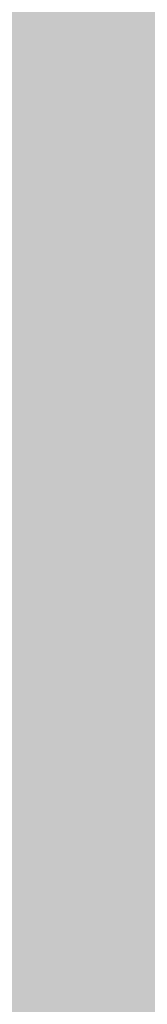
# Model space of a CAD drawing. Units: inches. Extents: x 2083 to 3317, y 1141 to 2115.
# Tile 217 of 256: x 3126.67 to 3126.939, y 1265.165 to 1267.234. Entities that reach past the tile are written whole.
import ezdxf

# ---------------------------------------------------------------- set-up
doc = ezdxf.new("R2010")
doc.units = ezdxf.units.IN
doc.layers.add('A-ANNO-DIMS', color=2, linetype='Continuous', lineweight=18)
doc.layers.add('A-WALL-PATT', color=251, linetype='Continuous', lineweight=13, true_color=0x636466)
doc.styles.get("Standard").update_dxf_attribs({"font": 'arial.ttf'})
doc.dimstyles.new('ISO-25', dxfattribs={"dimtxt": 12, "dimasz": 12, "dimexe": 1.25, "dimexo": 0.625, "dimtad": 1, "dimlunit": 3, "dimtxsty": 'Standard', "dimcen": 2.5, "dimadec": 0, "dimazin": 0, "dimtfac": 1, "dimtmove": 0, "dimatfit": 3, "dimfxl": 1, "dimarcsym": 0})

# ---------------------------------------------------------------- blocks, each defined once
blk = doc.blocks.new('*D26')
at = {"layer": 'A-ANNO-DIMS', "color": 0, "lineweight": -2, "transparency": 16777216}
for p, q in [((3088.9858, 1274.9151), (3088.9858, 1270.952)), ((3111.24, 1274.9151), (3111.24, 1270.952)), ((3076.9858, 1272.202), (2840.2624, 1272.202)), ((3111.24, 1272.202), (3088.9858, 1272.202)), ((3123.24, 1272.202), (3135.24, 1272.202))]:
    blk.add_line(p, q, dxfattribs=at)
at = {"layer": 'A-ANNO-DIMS', "color": 0, "transparency": 16777216}
for points in [[(3076.9858, 1274.202), (3076.9858, 1270.202), (3088.9858, 1272.202)], [(3123.24, 1274.202), (3123.24, 1270.202), (3111.24, 1272.202)]]:
    blk.add_solid(points, dxfattribs=at)
at = {"layer": 'Defpoints', "color": 0, "transparency": 16777216}
for p in [(3088.9858, 1275.5401), (3111.24, 1275.5401), (3088.9858, 1272.202)]:
    blk.add_point(p, dxfattribs=at)
at = {"layer": 'A-ANNO-DIMS', "color": 0, "transparency": 16777216, "insert": (2952.6241, 1279.0316), "char_height": 12, "attachment_point": 5}
blk.add_mtext('NIGHTSTAND 1\'-10 1/2" TYP.', dxfattribs=at)
blk = doc.blocks.new('*D27')
at = {"layer": 'A-ANNO-DIMS', "color": 0, "lineweight": -2, "transparency": 16777216}
for p, q in [((3114.5782, 1309.7943), (3114.5782, 1321.7943)), ((3111.865, 1297.7943), (3115.8282, 1297.7943)), ((3114.5782, 1297.7943), (3114.5782, 1275.5401)), ((3111.865, 1275.5401), (3115.8282, 1275.5401)), ((3114.5782, 1263.5401), (3114.5782, 1140.9886))]:
    blk.add_line(p, q, dxfattribs=at)
at = {"layer": 'A-ANNO-DIMS', "color": 0, "transparency": 16777216}
for points in [[(3112.5782, 1309.7943), (3116.5782, 1309.7943), (3114.5782, 1297.7943)], [(3112.5782, 1263.5401), (3116.5782, 1263.5401), (3114.5782, 1275.5401)]]:
    blk.add_solid(points, dxfattribs=at)
at = {"layer": 'Defpoints', "color": 0, "transparency": 16777216}
for p in [(3111.24, 1297.7943), (3111.24, 1275.5401), (3114.5782, 1275.5401)]:
    blk.add_point(p, dxfattribs=at)
at = {"layer": 'A-ANNO-DIMS', "color": 0, "transparency": 16777216, "insert": (3107.7485, 1196.2643), "char_height": 12, "attachment_point": 5, "rotation": 90}
blk.add_mtext('1\'-10 1/2" TYP.', dxfattribs=at)

msp = doc.modelspace()

# ---------------------------------------------------------------- hatches: boundary and pattern name
at = {"layer": 'A-WALL-PATT'}
h = msp.add_hatch(color=256, dxfattribs=at)
h.dxf.hatch_style = 1
h.paths.add_polyline_path([(3126.9598, 2020.7614), (2748.9598, 2020.7614), (2604.9598, 2020.7614), (2226.9598, 2020.7614), (2226.9598, 1702.7614), (2466.9598, 1702.7614), (2466.9598, 1582.7614), (2418.9598, 1582.7614), (2418.9598, 1477.7614), (2226.9598, 1477.7614), (2226.9598, 1263.2614), (2544.9598, 1263.2614), (2544.9598, 1411.7614), (2604.9598, 1411.7614), (2685.9598, 1411.7614), (2685.9598, 1420.7614), (2604.9598, 1420.7614), (2604.9598, 1573.7614), (2604.9598, 1702.7614), (2604.9598, 2011.7614), (2748.9598, 2011.7614), (2748.9598, 1702.7614), (2862.9598, 1702.7614), (2862.9598, 1621.7614), (2871.9598, 1621.7614), (2871.9598, 1702.7614), (2883.9598, 1702.7614), (2883.9598, 1706.9395, -0.026459), (2883.9598, 1711.7614), (2757.9598, 1711.7614), (2757.9598, 1807.7614), (2787.9598, 1807.7614), (2787.9598, 1812.2614), (2757.9598, 1812.2614), (2757.9598, 2011.7614), (2877.9598, 2011.7614), (2877.9598, 1812.2614), (2847.9598, 1812.2614), (2847.9598, 1807.7614), (2889.8357, 1807.7614), (2889.8357, 1812.2614), (2882.4598, 1812.2614), (2882.4598, 2011.7614), (3117.9598, 2011.7614), (3117.9598, 1812.2614), (2937.8357, 1812.2614), (2937.8357, 1807.7614), (2995.7098, 1807.7614), (2995.7098, 1796.1177), (3000.2098, 1796.1177), (3000.2098, 1807.7614), (3117.9598, 1807.7614), (3117.9598, 1711.7614), (3000.2098, 1711.7614), (3000.2098, 1760.1177), (2998.5727, 1760.1177, -0.020711), (2995.7098, 1760.1177), (2995.7098, 1711.7614), (2931.9598, 1711.7614), (2931.9598, 1702.7614), (3126.9598, 1702.7614)])
h.paths.add_polyline_path([(2471.4598, 2011.7614), (2471.4598, 1810.0114), (2462.7169, 1810.0114), (2462.7169, 1805.5114), (2505.9598, 1805.5114), (2505.9598, 1810.0114), (2475.9598, 1810.0114), (2475.9598, 2011.7614), (2595.9598, 2011.7614), (2595.9598, 1810.0114), (2565.9598, 1810.0114), (2565.9598, 1805.5114), (2595.9598, 1805.5114), (2595.9598, 1711.7614), (2235.9598, 1711.7614), (2235.9598, 1805.5114), (2353.7098, 1805.5114), (2353.7098, 1796.0542), (2358.2098, 1796.0542), (2358.2098, 1805.5114), (2414.7169, 1805.5114), (2414.7169, 1810.0114), (2235.9598, 1810.0114), (2235.9598, 2011.7614)], flags=16)
h.paths.add_polyline_path([(2270.2047, 1994.61), (2270.2047, 1970.61), (2246.2047, 1970.61), (2246.2047, 1994.61)], flags=0)
edge = h.paths.add_edge_path(flags=0)
edge.add_ellipse((2332.0274, 1899.7982), major_axis=(-3.043, 3.043), ratio=0.168252, start_angle=-161.3322, end_angle=-156.3071, ccw=False)
edge.add_ellipse((2333.082, 1898.7435), major_axis=(-1.0546, 1.0546), ratio=0.453532, start_angle=-123.371, end_angle=-94.1591)
edge = h.paths.add_edge_path(flags=0)
edge.add_ellipse((2332.0274, 1968.8763), major_axis=(3.043, 3.043), ratio=0.168252, start_angle=18.6678, end_angle=23.6929)
edge.add_spline(control_points=[(2332.9256, 1970.6911), (2332.2268, 1970.3361), (2330.8937, 1969.6589), (2328.4131, 1970.9321), (2327.2039, 1967.7487), (2324.7096, 1969.9556), (2322.5328, 1967.0124), (2320.0128, 1971.2958), (2317.6803, 1968.1578), (2316.0405, 1967.102), (2315.4269, 1966.8096)], knot_values=[0, 0, 0, 0, 2.267059, 4.324559, 6.685584, 8.878641, 11.121502, 14.300359, 17.755284, 19.732645, 19.732645, 19.732645, 19.732645], degree=3, periodic=0)
edge.add_ellipse((2332.0274, 1968.8763), major_axis=(3.043, 3.043), ratio=0.168252, start_angle=18.6678, end_angle=23.6929, ccw=False)
edge.add_ellipse((2333.082, 1969.9309), major_axis=(1.0546, 1.0546), ratio=0.453532, start_angle=56.629, end_angle=85.8409, ccw=False)
edge = h.paths.add_edge_path(flags=0)
edge.add_spline(control_points=[(2296.4283, 1967.9879), (2293.6278, 1965.3363), (2287.7036, 1959.7271), (2299.7439, 1949.9957), (2294.5326, 1935.6685), (2290.5732, 1920.6035), (2293.3941, 1909.9737), (2296.1854, 1904.9665)], knot_values=[0.099185, 0.099185, 0.099185, 0.099185, 0.345301, 0.619822, 0.982653, 1.386093, 1.810555, 1.810555, 1.810555, 1.810555], degree=3, periodic=0)
edge.add_spline(control_points=[(2296.1854, 1904.9665), (2297.3836, 1902.6193), (2298.001, 1901.9493), (2298.553, 1901.4682)], knot_values=[0.006246, 0.006246, 0.006246, 0.006246, 0.055476, 0.055476, 0.055476, 0.055476], degree=3, periodic=0)
edge.add_spline(control_points=[(2298.553, 1901.4682), (2297.2586, 1900.9232), (2295.2253, 1900.2321), (2293.0602, 1900.6142), (2292.1014, 1900.7884), (2292.0896, 1900.7906)], knot_values=[0.312835, 0.312835, 0.312835, 0.312835, 0.40178, 0.474987, 0.475903, 0.475903, 0.475903, 0.475903], degree=3, periodic=0)
edge.add_arc((2292.7936, 1904.6641), 3.937, 215.4209, 259.6982, ccw=False)
edge.add_spline(control_points=[(2289.5853, 1902.3823), (2289.4767, 1902.5351), (2289.3685, 1902.688), (2289.2609, 1902.8412)], knot_values=[0.102872, 0.102872, 0.102872, 0.102872, 0.116896, 0.116896, 0.116896, 0.116896], degree=3, periodic=0)
edge.add_spline(control_points=[(2289.2609, 1902.8412), (2288.6866, 1902.5502), (2287.64, 1902.0199), (2285.8813, 1901.874), (2283.853, 1901.5044), (2281.72, 1899.7105), (2278.467, 1899.4929), (2276.1571, 1901.8832), (2272.259, 1899.8041), (2267.7776, 1901.8432), (2262.2439, 1900.184), (2257.4149, 1901.7821), (2254.3184, 1900.7261), (2253.1783, 1900.3373)], knot_values=[0, 0, 0, 0, 1.907977, 3.477176, 5.261074, 7.972851, 11.680248, 13.717921, 16.939592, 22.789562, 27.502503, 33.595215, 37.145618, 37.145618, 37.145618, 37.145618], degree=3, periodic=0)
edge.add_line((2253.1783, 1900.3373), (2250.2442, 1902.8412))
edge.add_line((2250.2442, 1902.8412), (2250.2442, 1965.8333))
edge.add_line((2250.2442, 1965.8333), (2253.1783, 1968.3371))
edge.add_spline(control_points=[(2253.1783, 1968.3371), (2254.3184, 1967.9483), (2257.4149, 1966.8924), (2262.2439, 1968.4904), (2267.7776, 1966.8313), (2271.5267, 1968.5372), (2273.8759, 1967.8283), (2274.2067, 1967.7276)], knot_values=[0, 0, 0, 0, 0.09018, 0.244935, 0.364644, 0.513233, 0.537855, 0.537855, 0.537855, 0.537855], degree=3, periodic=0)
edge.add_arc((2274.3529, 1963.7933), 3.937, 72.0511, 92.1279, ccw=False)
edge.add_arc((2281.2969, 1985.23), 18.5963, 252.05113, 288.56572)
edge.add_arc((2292.3167, 1956.0289), 12.6461, 71.02679, 113.77822, ccw=False)
edge = h.paths.add_edge_path(flags=0)
edge.add_spline(control_points=[(2274.8994, 1951.8562), (2275.0662, 1951.6166), (2275.2327, 1951.3766), (2275.398, 1951.1359)], knot_values=[1.409916, 1.409916, 1.409916, 1.409916, 1.43159, 1.43159, 1.43159, 1.43159], degree=3, periodic=0)
edge.add_spline(control_points=[(2275.398, 1951.1359), (2275.7921, 1950.5619), (2276.1792, 1949.9838), (2276.5455, 1949.3971)], knot_values=[1.358238, 1.358238, 1.358238, 1.358238, 1.409916, 1.409916, 1.409916, 1.409916], degree=3, periodic=0)
edge.add_line((2276.5455, 1949.3971), (2277.4373, 1947.8622))
edge.add_spline(control_points=[(2277.4373, 1947.8622), (2276.3038, 1945.6731), (2274.6397, 1942.4269), (2274.6316, 1938.0939), (2272.7991, 1930.8515), (2274.3564, 1943.897), (2275.9477, 1947.9234), (2276.5455, 1949.3971)], knot_values=[0.005632, 0.005632, 0.005632, 0.005632, 0.186014, 0.266002, 0.357087, 0.59639, 0.739732, 0.739732, 0.739732, 0.739732], degree=3, periodic=0)
edge.add_spline(control_points=[(2276.5455, 1949.3971), (2276.1792, 1949.9838), (2275.7921, 1950.5619), (2275.398, 1951.1359)], knot_values=[1.358238, 1.358238, 1.358238, 1.358238, 1.409916, 1.409916, 1.409916, 1.409916], degree=3, periodic=0)
edge.add_spline(control_points=[(2275.398, 1951.1359), (2274.9425, 1950.0805), (2274.2078, 1948.0253), (2273.9346, 1944.8515), (2272.4685, 1937.6275), (2273.4662, 1945.6965), (2274.7006, 1951.0595), (2274.8994, 1951.8562)], knot_values=[0.104364, 0.104364, 0.104364, 0.104364, 0.189636, 0.269624, 0.36071, 0.600013, 0.644622, 0.644622, 0.644622, 0.644622], degree=3, periodic=0)
h.paths.add_polyline_path([(2269.1675, 1963.1276, -0.357527), (2268.1706, 1960.9764, -0.092561), (2268.1706, 1939.4363, -0.357527), (2269.1675, 1937.2851, -0.357527), (2267.0163, 1938.282, -0.164785), (2254.6856, 1938.282, -0.357527), (2252.5344, 1937.2851, -0.357527), (2253.5313, 1939.4363, -0.092561), (2253.5313, 1960.9764, -0.357527), (2252.5344, 1963.1276, -0.357527), (2254.6856, 1962.1307, -0.164785), (2267.0163, 1962.1307, -0.357527)], flags=0)
h.paths.add_polyline_path([(2248.8741, 1967.8018), (2248.8741, 1957.0277), (2249.4578, 1957.0277), (2249.4578, 1911.6468), (2248.8741, 1911.6468), (2248.8741, 1900.8727), (2246.5119, 1900.8727, 0.197327), (2244.1497, 1902.4569), (2244.1497, 1966.2176, 0.197327), (2246.5119, 1967.8018)], flags=0)
h.paths.add_polyline_path([(2269.1675, 1931.3893, -0.357527), (2268.1706, 1929.2381, -0.092561), (2268.1706, 1907.6981, -0.357527), (2269.1675, 1905.5469, -0.357527), (2267.0163, 1906.5438, -0.164785), (2254.6856, 1906.5438, -0.357527), (2252.5344, 1905.5469, -0.357527), (2253.5313, 1907.6981, -0.092561), (2253.5313, 1929.2381, -0.357527), (2252.5344, 1931.3893, -0.357527), (2254.6856, 1930.3925, -0.164785), (2267.0163, 1930.3925, -0.357527)], flags=0)
edge = h.paths.add_edge_path(flags=0)
edge.add_spline(control_points=[(2276.1969, 1906.7237), (2276.1681, 1909.0289), (2276.114, 1913.3719), (2270.5984, 1924.925), (2273.9052, 1919.0128), (2275.9217, 1916.2621), (2275.4746, 1912.4021), (2277.2579, 1910.3806), (2276.696, 1908.225), (2276.6462, 1906.813), (2276.6178, 1906.0084)], knot_values=[0, 0, 0, 0, 8.61026, 16.221274, 18.843057, 23.804898, 27.440828, 29.356102, 31.203478, 33.650687, 33.650687, 33.650687, 33.650687], degree=3, periodic=0)
edge.add_spline(control_points=[(2276.6178, 1906.0084), (2276.6233, 1905.6241), (2276.4977, 1904.6287), (2275.4418, 1903.8547), (2274.9373, 1903.0804), (2274.8591, 1902.8412)], knot_values=[0.156488, 0.156488, 0.156488, 0.156488, 0.184398, 0.231376, 0.250598, 0.250598, 0.250598, 0.250598], degree=3, periodic=0)
edge.add_line((2274.8591, 1902.8412), (2276.506, 1902.8412))
edge.add_spline(control_points=[(2276.506, 1902.8412), (2276.7883, 1903.0849), (2277.6651, 1904.1252), (2278.2495, 1904.3407), (2277.6539, 1908.5274), (2278.1557, 1906.2278), (2278.1005, 1905.2859), (2278.8467, 1904.069), (2277.8568, 1903.4149), (2277.8742, 1902.991), (2277.9036, 1902.8412)], knot_values=[0.059574, 0.059574, 0.059574, 0.059574, 0.080753, 0.103741, 0.16972, 0.176036, 0.207137, 0.240474, 0.262341, 0.27366, 0.27366, 0.27366, 0.27366], degree=3, periodic=0)
edge.add_line((2277.9036, 1902.8412), (2280.0298, 1902.8412))
edge.add_spline(control_points=[(2280.0298, 1902.8412), (2279.8882, 1903.0884), (2279.4993, 1903.9816), (2280.1523, 1905.9393), (2278.1036, 1909.6578), (2279.7624, 1907.1853), (2280.3279, 1904.8749), (2280.4851, 1903.4896), (2281.4633, 1903.2494), (2281.7583, 1902.9365), (2281.834, 1902.8412)], knot_values=[0.013856, 0.013856, 0.013856, 0.013856, 0.034874, 0.088867, 0.107879, 0.126738, 0.158714, 0.193757, 0.217487, 0.226722, 0.226722, 0.226722, 0.226722], degree=3, periodic=0)
edge.add_spline(control_points=[(2281.834, 1902.8412), (2281.7875, 1902.8267), (2281.647, 1902.783), (2281.3955, 1902.8595), (2281.0881, 1902.9852), (2280.7207, 1903.0609), (2280.3335, 1903.0257), (2280.1248, 1902.8989), (2280.0298, 1902.8412)], knot_values=[0, 0, 0, 0, 0.14413, 0.435517, 0.749276, 1.153046, 1.548371, 1.878348, 1.878348, 1.878348, 1.878348], degree=3, periodic=0)
edge.add_line((2280.0298, 1902.8412), (2277.9036, 1902.8412))
edge.add_spline(control_points=[(2277.9036, 1902.8412), (2277.8929, 1902.7959), (2277.8654, 1902.6796), (2277.6075, 1902.6875), (2277.2741, 1902.8007), (2276.8379, 1902.6198), (2276.5838, 1902.7893), (2276.506, 1902.8412)], knot_values=[0, 0, 0, 0, 0.127189, 0.326199, 0.628009, 1.24357, 1.515331, 1.515331, 1.515331, 1.515331], degree=3, periodic=0)
edge.add_line((2276.506, 1902.8412), (2274.8591, 1902.8412))
edge.add_spline(control_points=[(2274.8591, 1902.8412), (2274.8144, 1902.8986), (2274.7251, 1903.0134), (2274.4935, 1903.119), (2274.2443, 1902.9605), (2273.9371, 1903.1849), (2273.614, 1902.9831), (2273.4083, 1902.883), (2273.3223, 1902.8412)], knot_values=[0, 0, 0, 0, 0.21843, 0.436957, 0.687977, 0.990379, 1.398396, 1.69185, 1.69185, 1.69185, 1.69185], degree=3, periodic=0)
edge.add_spline(control_points=[(2273.3223, 1902.8412), (2273.6167, 1903.4457), (2274.274, 1904.5383), (2276.0272, 1904.5737), (2276.207, 1906.5836), (2276.1969, 1906.7237)], knot_values=[0.012227, 0.012227, 0.012227, 0.012227, 0.059472, 0.106218, 0.134458, 0.134458, 0.134458, 0.134458], degree=3, periodic=0)
h.paths.add_polyline_path([(2270.7761, 1897.7898), (2270.7761, 1873.7898), (2246.7761, 1873.7898), (2246.7761, 1897.7898)], flags=0)
h.paths.add_polyline_path([(2353.7098, 1760.0051), (2353.7098, 1760.0542), (2358.2098, 1760.0542, -0.033729)], flags=0)
h.paths.add_polyline_path([(2321.8191, 1737.5292), (2341.9953, 1737.5292, -0.414214), (2343.2033, 1736.3212), (2343.2033, 1721.0206, -0.414214), (2341.9953, 1719.8127), (2321.8191, 1719.8127, -0.414214), (2320.6112, 1721.0206), (2320.6112, 1736.3212, -0.414214)], flags=0)
h.paths.add_polyline_path([(2324.235, 1736.3212), (2339.5794, 1736.3212, -0.414214), (2341.9953, 1733.9053), (2341.9953, 1725.4497, -0.414214), (2339.5794, 1723.0338), (2333.6806, 1723.0338), (2333.8453, 1722.0455, -0.870646), (2335.4254, 1721.8259, -0.767327), (2333.9227, 1721.4232), (2331.291, 1721.4232, -0.767327), (2329.7883, 1721.8259, -0.870646), (2331.3684, 1722.0455), (2331.5331, 1723.0338), (2324.235, 1723.0338, -0.414214), (2321.8191, 1725.4497), (2321.8191, 1733.9053, -0.414214)], flags=0)
h.paths.add_polyline_path([(2570.4838, 1928.6154), (2589.6838, 1928.6154), (2590.1688, 1928.6154), (2590.1688, 1904.9934), (2570.4838, 1904.9934)], flags=0)
h.paths.add_polyline_path([(2574.4473, 1927.2638, -1), (2572.8288, 1927.2638, -1)], flags=0)
h.paths.add_polyline_path([(2573.0899, 1926.9409), (2573.925, 1927.776), (2574.1477, 1927.5533), (2573.3126, 1926.7182)], flags=0)
h.paths.add_polyline_path([(2578.7791, 1919.7296, -1), (2571.5917, 1919.7296, -1)], flags=0)
h.paths.add_polyline_path([(2578.3854, 1919.7296, -1), (2571.9854, 1919.7296, -1)], flags=0)
h.paths.add_polyline_path([(2331.5958, 1729.4762, -1), (2333.618, 1729.4762, -1)], flags=0)
h.paths.add_polyline_path([(2578.0342, 1927.2638, -1), (2576.4157, 1927.2638, -1)], flags=0)
h.paths.add_polyline_path([(2576.6889, 1927.5311), (2576.9116, 1927.7538), (2577.7467, 1926.9186), (2577.524, 1926.6959)], flags=0)
h.paths.add_polyline_path([(2578.1391, 1909.8595, -1), (2572.2317, 1909.8595, -1)], flags=0)
h.paths.add_polyline_path([(2577.7454, 1909.8595, -1), (2572.6254, 1909.8595, -1)], flags=0)
h.paths.add_polyline_path([(2583.7977, 1927.2638, -1), (2582.1792, 1927.2638, -1)], flags=0)
h.paths.add_polyline_path([(2582.7186, 1927.7538), (2583.5538, 1926.9186), (2583.3311, 1926.6959), (2582.4959, 1927.5311)], flags=0)
h.paths.add_polyline_path([(2582.4959, 1927.5311), (2582.7186, 1927.7538), (2583.5538, 1926.9186), (2583.3311, 1926.6959)], flags=0)
h.paths.add_polyline_path([(2587.7391, 1920.5296, -1), (2581.8317, 1920.5296, -1)], flags=0)
h.paths.add_polyline_path([(2587.3454, 1920.5296, -1), (2582.2254, 1920.5296, -1)], flags=0)
h.paths.add_polyline_path([(2587.3846, 1927.2638, -1), (2585.7661, 1927.2638, -1)], flags=0)
h.paths.add_polyline_path([(2586.082, 1926.9802), (2586.9172, 1927.8154), (2587.1399, 1927.5927), (2586.3047, 1926.7575)], flags=0)
h.paths.add_polyline_path([(2588.3791, 1910.6595, -1), (2581.1917, 1910.6595, -1)], flags=0)
h.paths.add_polyline_path([(2587.9854, 1910.6595, -1), (2581.5854, 1910.6595, -1)], flags=0)
h.paths.add_polyline_path([(2417.1677, 1729.4779), (2437.3439, 1729.4779, -0.414214), (2438.5519, 1728.2699), (2438.5519, 1712.9693, -0.414214), (2437.3439, 1711.7614), (2417.1677, 1711.7614, -0.414214), (2415.9598, 1712.9693), (2415.9598, 1728.2699, -0.414214)], flags=0)
h.paths.add_polyline_path([(2419.5836, 1728.2699), (2434.928, 1728.2699, -0.414214), (2437.3439, 1725.8541), (2437.3439, 1717.3984, -0.414214), (2434.928, 1714.9825), (2429.0292, 1714.9825), (2429.1939, 1713.9942, -0.870646), (2430.774, 1713.7746, -0.767327), (2429.2713, 1713.372), (2426.6396, 1713.372, -0.767327), (2425.1369, 1713.7746, -0.870646), (2426.717, 1713.9942), (2426.8817, 1714.9825), (2419.5836, 1714.9825, -0.414214), (2417.1677, 1717.3984), (2417.1677, 1725.8541, -0.414214)], flags=0)
h.paths.add_polyline_path([(2419.5836, 1728.2699), (2434.928, 1728.2699, -0.414214), (2437.3439, 1725.8541), (2437.3439, 1717.3984, -0.414214), (2434.928, 1714.9825), (2429.0292, 1714.9825), (2428.3581, 1719.009), (2427.5528, 1719.009), (2426.8817, 1714.9825), (2419.5836, 1714.9825, -0.414214), (2417.1677, 1717.3984), (2417.1677, 1725.8541, -0.414214)], flags=0)
h.paths.add_polyline_path([(2426.9444, 1721.4249, -1), (2428.9666, 1721.4249, -1)], flags=0)
h.paths.add_polyline_path([(2475.9598, 1702.7614), (2595.9598, 1702.7614), (2595.9598, 1582.7614), (2475.9598, 1582.7614)], flags=16)
h.paths.add_polyline_path([(2427.9598, 1573.7614), (2595.9598, 1573.7614), (2595.9598, 1468.7614), (2595.9598, 1420.7614), (2384.4598, 1420.7614), (2384.4598, 1468.7614), (2427.9598, 1468.7614)], flags=16)
h.paths.add_polyline_path([(2379.9598, 1468.7614), (2379.9598, 1420.7614), (2235.9598, 1420.7614), (2235.9598, 1468.7614)], flags=16)
h.paths.add_polyline_path([(2317.816, 1466.6958), (2337.9922, 1466.6958, -0.414214), (2339.2002, 1465.4878), (2339.2002, 1450.1872, -0.414214), (2337.9922, 1448.9792), (2317.816, 1448.9792, -0.414214), (2316.6081, 1450.1872), (2316.6081, 1465.4878, -0.414214)], flags=0)
h.paths.add_polyline_path([(2320.2319, 1465.4878), (2335.5763, 1465.4878, -0.414214), (2337.9922, 1463.0719), (2337.9922, 1454.6163, -0.414214), (2335.5763, 1452.2004), (2329.6775, 1452.2004), (2329.8422, 1451.212, -0.870646), (2331.4223, 1450.9925, -0.767327), (2329.9196, 1450.5898), (2327.2879, 1450.5898, -0.767327), (2325.7852, 1450.9925, -0.870646), (2327.3653, 1451.212), (2327.53, 1452.2004), (2320.2319, 1452.2004, -0.414214), (2317.816, 1454.6163), (2317.816, 1463.0719, -0.414214)], flags=0)
h.paths.add_polyline_path([(2320.2319, 1465.4878), (2335.5763, 1465.4878, -0.414214), (2337.9922, 1463.0719), (2337.9922, 1454.6163, -0.414214), (2335.5763, 1452.2004), (2329.6775, 1452.2004), (2329.0064, 1456.2269), (2328.2011, 1456.2269), (2327.53, 1452.2004), (2320.2319, 1452.2004, -0.414214), (2317.816, 1454.6163), (2317.816, 1463.0719, -0.414214)], flags=0)
h.paths.add_polyline_path([(2327.5926, 1458.6428, -1), (2329.6148, 1458.6428, -1)], flags=0)
h.paths.add_polyline_path([(2244.4117, 1433.3405), (2241.9209, 1433.3405, -0.414214), (2240.0179, 1435.2435), (2240.0179, 1440.9528, -0.414211), (2241.9209, 1442.8559), (2244.4117, 1442.8559, -1.976472)], flags=0)
h.paths.add_polyline_path([(2245.3569, 1434.3975, -0.414214), (2245.3569, 1441.7988, -2.144098)], flags=0)
h.paths.add_polyline_path([(2535.9598, 1416.2614), (2535.9598, 1272.2614), (2235.9598, 1272.2614), (2235.9598, 1416.2614)], flags=16)
h.paths.add_polyline_path([(2260.1196, 1384.2928), (2260.1196, 1362.0386), (2237.8654, 1362.0386), (2237.8654, 1384.2928)], flags=0)
edge = h.paths.add_edge_path(flags=0)
edge.add_line((2318.2518, 1362.0933), (2318.1458, 1362.001))
edge.add_ellipse((2317.4451, 1360.431), major_axis=(2.8216, 2.8216), ratio=0.168252, start_angle=18.6678, end_angle=20.9481, ccw=False)
edge.add_ellipse((2318.423, 1361.409), major_axis=(0.9779, 0.9779), ratio=0.453532, start_angle=56.629, end_angle=70.2262, ccw=False)
edge = h.paths.add_edge_path(flags=0)
edge.add_line((2319.1074, 1295.5711), (2319.015, 1295.6771))
edge.add_ellipse((2317.4451, 1296.3778), major_axis=(-2.8216, 2.8216), ratio=0.168252, start_angle=-161.3322, end_angle=-159.0519, ccw=False)
edge.add_ellipse((2318.423, 1295.3999), major_axis=(-0.9779, 0.9779), ratio=0.453532, start_angle=-123.371, end_angle=-109.7738)
edge = h.paths.add_edge_path(flags=0)
edge.add_spline(control_points=[(2284.2103, 1301.1702), (2284.5807, 1300.4447), (2284.8912, 1299.892), (2285.1596, 1299.461)], knot_values=[0.039066, 0.039066, 0.039066, 0.039066, 0.055476, 0.055476, 0.055476, 0.055476], degree=3, periodic=0)
edge.add_line((2285.1596, 1299.461), (2284.2103, 1301.1702))
edge = h.paths.add_edge_path(flags=0)
edge.add_line((2280.4125, 1297.298), (2283.37, 1297.0361))
edge.add_line((2283.37, 1297.0361), (2286.4057, 1297.9263))
edge.add_spline(control_points=[(2286.4057, 1297.9263), (2285.3055, 1297.4631), (2284.3448, 1297.1292), (2283.37, 1297.0361)], knot_values=[0.394369, 0.394369, 0.394369, 0.394369, 0.475903, 0.475903, 0.475903, 0.475903], degree=3, periodic=0)
edge.add_spline(control_points=[(2283.37, 1297.0361), (2283.2814, 1297.0277), (2282.3163, 1296.9573), (2281.3125, 1297.1345), (2280.4234, 1297.296), (2280.4125, 1297.298)], knot_values=[0.312835, 0.312835, 0.312835, 0.312835, 0.320246, 0.393453, 0.394369, 0.394369, 0.394369, 0.394369], degree=3, periodic=0)
edge = h.paths.add_edge_path(flags=0)
edge.add_line((2284.4356, 1359.6073), (2280.4463, 1355.328))
edge.add_line((2280.4463, 1355.328), (2279.58, 1351.0178))
edge.add_line((2279.58, 1351.0178), (2282.413, 1346.5804))
edge.add_spline(control_points=[(2282.413, 1346.5804), (2283.1533, 1345.5892), (2284.2529, 1344.0289), (2284.801, 1342.3872), (2284.9352, 1341.8055)], knot_values=[1.240098, 1.240098, 1.240098, 1.240098, 1.332892, 1.382712, 1.382712, 1.382712, 1.382712], degree=3, periodic=0)
edge.add_spline(control_points=[(2284.9352, 1341.8055), (2285.3191, 1340.1406), (2285.233, 1338.4092), (2284.9099, 1336.6541)], knot_values=[1.097484, 1.097484, 1.097484, 1.097484, 1.240098, 1.240098, 1.240098, 1.240098], degree=3, periodic=0)
edge.add_spline(control_points=[(2284.9099, 1336.6541), (2284.5868, 1334.899), (2284.0267, 1333.1203), (2283.4626, 1331.3606)], knot_values=[0.95487, 0.95487, 0.95487, 0.95487, 1.097484, 1.097484, 1.097484, 1.097484], degree=3, periodic=0)
edge.add_line((2283.4626, 1331.3606), (2281.8904, 1326.1534))
edge.add_line((2281.8904, 1326.1534), (2280.7563, 1321.0561))
edge.add_line((2280.7563, 1321.0561), (2280.2992, 1316.002))
edge.add_line((2280.2992, 1316.002), (2280.7159, 1310.9501))
edge.add_line((2280.7159, 1310.9501), (2282.0281, 1305.9721))
edge.add_line((2282.0281, 1305.9721), (2284.2103, 1301.1702))
edge.add_spline(control_points=[(2284.2103, 1301.1702), (2283.3407, 1302.7302), (2282.6119, 1304.3365), (2282.0281, 1305.9721)], knot_values=[0.099185, 0.099185, 0.099185, 0.099185, 0.241799, 0.241799, 0.241799, 0.241799], degree=3, periodic=0)
edge.add_spline(control_points=[(2282.0281, 1305.9721), (2281.4443, 1307.6078), (2281.0055, 1309.2728), (2280.7159, 1310.9501)], knot_values=[0.241799, 0.241799, 0.241799, 0.241799, 0.384413, 0.384413, 0.384413, 0.384413], degree=3, periodic=0)
edge.add_spline(control_points=[(2280.7159, 1310.9501), (2280.4332, 1312.5876), (2280.2894, 1314.277), (2280.2989, 1315.962), (2280.2992, 1316.002)], knot_values=[0.384413, 0.384413, 0.384413, 0.384413, 0.523647, 0.527028, 0.527028, 0.527028, 0.527028], degree=3, periodic=0)
edge.add_spline(control_points=[(2280.2992, 1316.002), (2280.3123, 1317.687), (2280.4779, 1319.3679), (2280.7563, 1321.0561)], knot_values=[0.527028, 0.527028, 0.527028, 0.527028, 0.669642, 0.669642, 0.669642, 0.669642], degree=3, periodic=0)
edge.add_spline(control_points=[(2280.7563, 1321.0561), (2281.0346, 1322.7443), (2281.4259, 1324.4396), (2281.8904, 1326.1534)], knot_values=[0.669642, 0.669642, 0.669642, 0.669642, 0.812256, 0.812256, 0.812256, 0.812256], degree=3, periodic=0)
edge.add_spline(control_points=[(2281.8904, 1326.1534), (2282.2644, 1327.5333), (2282.7879, 1329.2618), (2283.3528, 1331.0178), (2283.4626, 1331.3606)], knot_values=[0.812256, 0.812256, 0.812256, 0.812256, 0.927087, 0.95487, 0.95487, 0.95487, 0.95487], degree=3, periodic=0)
edge.add_line((2283.4626, 1331.3606), (2284.9099, 1336.6541))
edge.add_line((2284.9099, 1336.6541), (2284.9352, 1341.8055))
edge.add_line((2284.9352, 1341.8055), (2282.413, 1346.5804))
edge.add_spline(control_points=[(2282.413, 1346.5804), (2281.2751, 1348.1038), (2280.0784, 1349.5703), (2279.58, 1351.0178)], knot_values=[1.382712, 1.382712, 1.382712, 1.382712, 1.525326, 1.525326, 1.525326, 1.525326], degree=3, periodic=0)
edge.add_spline(control_points=[(2279.58, 1351.0178), (2279.4433, 1351.4147), (2279.1363, 1352.8569), (2279.7352, 1354.2904), (2280.4463, 1355.328)], knot_values=[1.525326, 1.525326, 1.525326, 1.525326, 1.564439, 1.667941, 1.667941, 1.667941, 1.667941], degree=3, periodic=0)
edge.add_spline(control_points=[(2280.4463, 1355.328), (2281.4261, 1356.7578), (2282.9308, 1358.1826), (2284.4356, 1359.6073)], knot_values=[1.667941, 1.667941, 1.667941, 1.667941, 1.810555, 1.810555, 1.810555, 1.810555], degree=3, periodic=0)
edge.add_arc((2280.6231, 1348.5182), 11.7262, 71.02679, 113.77822)
edge.add_arc((2270.4049, 1375.5952), 17.2436, 252.05113, 288.56572, ccw=False)
edge.add_arc((2263.966, 1355.7178), 3.6506, 72.0511, 92.1279)
edge.add_arc((2263.966, 1355.7178), 3.6506, 92.1279, 177.9851)
edge.add_spline(control_points=[(2260.3176, 1355.8462), (2260.2604, 1354.2207), (2260.5513, 1350.1865), (2262.9993, 1346.7663), (2264.4727, 1344.649)], knot_values=[1.43159, 1.43159, 1.43159, 1.43159, 1.564144, 1.770695, 1.770695, 1.770695, 1.770695], degree=3, periodic=0)
edge.add_line((2264.4727, 1344.649), (2264.9356, 1343.9825))
edge.add_spline(control_points=[(2263.801, 1340.2481), (2263.8432, 1340.5141), (2264.0672, 1341.7565), (2264.5127, 1343.0025), (2264.935, 1343.9811)], knot_values=[0.53657, 0.53657, 0.53657, 0.53657, 0.559349, 0.644622, 0.644622, 0.644622, 0.644622], degree=3, periodic=0)
edge.add_spline(control_points=[(2264.935, 1343.9811), (2265.1178, 1343.715), (2265.2989, 1343.4479), (2265.4768, 1343.1794)], knot_values=[1.384077, 1.384077, 1.384077, 1.384077, 1.409916, 1.409916, 1.409916, 1.409916], degree=3, periodic=0)
edge.add_spline(control_points=[(2265.4768, 1343.1794), (2265.6546, 1342.9108), (2265.8293, 1342.6408), (2265.9991, 1342.3688)], knot_values=[1.358238, 1.358238, 1.358238, 1.358238, 1.384077, 1.384077, 1.384077, 1.384077], degree=3, periodic=0)
edge.add_line((2265.9991, 1342.3688), (2266.826, 1340.9455))
edge.add_spline(control_points=[(2266.826, 1340.9455), (2268.8944, 1337.0897), (2271.3982, 1325.843), (2270.5162, 1310.5686), (2275.9194, 1301.8606), (2277.7895, 1299.1994)], knot_values=[0.116896, 0.116896, 0.116896, 0.116896, 0.472987, 1.050969, 1.313793, 1.313793, 1.313793, 1.313793], degree=3, periodic=0)
edge.add_spline(control_points=[(2277.7895, 1299.1994), (2277.8394, 1299.1285), (2277.8894, 1299.0575), (2277.9396, 1298.9866)], knot_values=[0.109884, 0.109884, 0.109884, 0.109884, 0.116896, 0.116896, 0.116896, 0.116896], degree=3, periodic=0)
edge.add_line((2277.9396, 1298.9866), (2277.7888, 1299.1991))
edge.add_spline(control_points=[(2277.7888, 1299.1991), (2277.2566, 1298.9294), (2276.2864, 1298.4379), (2275.0394, 1298.3344), (2274.3833, 1298.2389), (2274.2153, 1298.2093)], knot_values=[33.12187, 33.12187, 33.12187, 33.12187, 35.029056, 36.598255, 37.144827, 37.144827, 37.144827, 37.144827], degree=3, periodic=0)
edge.add_line((2274.2153, 1298.2093), (2273.0731, 1297.893))
edge.add_spline(control_points=[(2273.0731, 1297.893), (2272.3229, 1297.5798), (2271.0392, 1296.5105), (2269.2484, 1296.2261), (2268.4231, 1296.3747)], knot_values=[26.532584, 26.532584, 26.532584, 26.532584, 29.198919, 31.839101, 31.839101, 31.839101, 31.839101], degree=3, periodic=0)
edge.add_line((2268.4231, 1296.3747), (2263.8785, 1297.4575))
edge.add_spline(control_points=[(2263.8785, 1297.4575), (2263.5561, 1297.3594), (2261.8603, 1296.8387), (2260.2388, 1297.2824), (2258.9335, 1297.5165)], knot_values=[15.919551, 15.919551, 15.919551, 15.919551, 16.939592, 21.226067, 21.226067, 21.226067, 21.226067], degree=3, periodic=0)
edge.add_line((2258.9335, 1297.5165), (2254.0552, 1297.329))
edge.add_spline(control_points=[(2254.0552, 1297.329), (2253.7555, 1297.2958), (2252.1137, 1297.1652), (2250.4619, 1297.5442), (2249.1297, 1297.6679)], knot_values=[5.306517, 5.306517, 5.306517, 5.306517, 6.276435, 10.613034, 10.613034, 10.613034, 10.613034], degree=3, periodic=0)
edge.add_line((2249.1297, 1297.6679), (2244.3316, 1296.8778))
edge.add_line((2244.3316, 1296.8778), (2241.611, 1299.1994))
edge.add_line((2241.611, 1299.1994), (2241.611, 1357.6094))
edge.add_line((2241.611, 1357.6094), (2244.3316, 1359.9311))
edge.add_line((2244.3316, 1359.9311), (2252.7288, 1359.5427))
edge.add_spline(control_points=[(2252.7288, 1359.5427), (2252.8709, 1359.5464), (2253.3057, 1359.5482), (2253.7398, 1359.5143), (2254.0317, 1359.4824)], knot_values=[0.233291, 0.233291, 0.233291, 0.233291, 0.244935, 0.268927, 0.268927, 0.268927, 0.268927], degree=3, periodic=0)
edge.add_line((2254.0317, 1359.4824), (2259.5872, 1359.4164))
edge.add_spline(control_points=[(2259.5872, 1359.4164), (2260.6771, 1359.6285), (2262.0732, 1359.897), (2263.5237, 1359.4593), (2263.8304, 1359.366)], knot_values=[0.422516, 0.422516, 0.422516, 0.422516, 0.513233, 0.537855, 0.537855, 0.537855, 0.537855], degree=3, periodic=0)
edge.add_arc((2263.966, 1355.7178), 3.6506, 72.0511, 92.1279, ccw=False)
edge.add_arc((2270.4049, 1375.5952), 17.2436, 252.05113, 288.56572)
edge.add_arc((2280.6231, 1348.5182), 11.7262, 71.02679, 113.77822, ccw=False)
h.paths.add_polyline_path([(2240.3405, 1359.4347), (2240.3405, 1349.4444), (2240.8818, 1349.4444), (2240.8818, 1307.3645), (2240.3405, 1307.3645), (2240.3405, 1297.3741), (2238.1502, 1297.3741, 0.197327), (2235.9598, 1298.8431), (2235.9598, 1357.9657, 0.197327), (2238.1502, 1359.4347)], flags=0)
h.paths.add_polyline_path([(2259.1578, 1355.1005, -0.357527), (2258.2334, 1353.1058, -0.092561), (2258.2334, 1333.1326, -0.357527), (2259.1578, 1331.1379, -0.357527), (2257.1631, 1332.0622, -0.164785), (2245.7293, 1332.0622, -0.357527), (2243.7346, 1331.1379, -0.357527), (2244.6589, 1333.1326, -0.092561), (2244.6589, 1353.1058, -0.357527), (2243.7346, 1355.1005, -0.357527), (2245.7293, 1354.1761, -0.164785), (2257.1631, 1354.1761, -0.357527)], flags=0)
edge = h.paths.add_edge_path(flags=0)
edge.add_line((2265.9991, 1342.3688), (2266.826, 1340.9455))
edge.add_line((2266.826, 1340.9455), (2265.3076, 1337.8141))
edge.add_line((2265.3076, 1337.8141), (2264.3582, 1334.6529))
edge.add_line((2264.3582, 1334.6529), (2264.262, 1333.7997))
edge.add_spline(control_points=[(2264.262, 1333.7997), (2264.2084, 1333.1871), (2264.1621, 1332.3655), (2264.0071, 1331.4139), (2263.969, 1331.2018)], knot_values=[0.464444, 0.464444, 0.464444, 0.464444, 0.516691, 0.531608, 0.531608, 0.531608, 0.531608], degree=3, periodic=0)
edge.add_spline(control_points=[(2263.969, 1331.2018), (2263.7745, 1330.1189), (2263.4244, 1328.7908), (2263.2574, 1328.5307), (2263.234, 1328.5146)], knot_values=[0.372682, 0.372682, 0.372682, 0.372682, 0.44885, 0.464444, 0.464444, 0.464444, 0.464444], degree=3, periodic=0)
edge.add_spline(control_points=[(2263.234, 1328.5146), (2263.0964, 1328.4202), (2263.1312, 1329.3015), (2263.275, 1330.6157)], knot_values=[0.280919, 0.280919, 0.280919, 0.280919, 0.372682, 0.372682, 0.372682, 0.372682], degree=3, periodic=0)
edge.add_spline(control_points=[(2263.275, 1330.6157), (2263.4187, 1331.93), (2263.6715, 1333.6773), (2263.9699, 1335.315)], knot_values=[0.189157, 0.189157, 0.189157, 0.189157, 0.280919, 0.280919, 0.280919, 0.280919], degree=3, periodic=0)
edge.add_spline(control_points=[(2263.9699, 1335.315), (2264.1005, 1336.0322), (2264.4188, 1337.6219), (2264.7548, 1338.8644), (2264.9474, 1339.4911)], knot_values=[0.097394, 0.097394, 0.097394, 0.097394, 0.137578, 0.189157, 0.189157, 0.189157, 0.189157], degree=3, periodic=0)
edge.add_spline(control_points=[(2264.9474, 1339.4911), (2265.29, 1340.6061), (2265.6442, 1341.494), (2265.9991, 1342.3688)], knot_values=[0.005632, 0.005632, 0.005632, 0.005632, 0.097394, 0.097394, 0.097394, 0.097394], degree=3, periodic=0)
h.paths.add_polyline_path([(2259.1578, 1325.671, -0.357527), (2258.2334, 1323.6763, -0.092561), (2258.2334, 1303.7031, -0.357527), (2259.1578, 1301.7084, -0.357527), (2257.1631, 1302.6327, -0.164785), (2245.7293, 1302.6327, -0.357527), (2243.7346, 1301.7084, -0.357527), (2244.6589, 1303.7031, -0.092561), (2244.6589, 1323.6763, -0.357527), (2243.7346, 1325.671, -0.357527), (2245.7293, 1324.7466, -0.164785), (2257.1631, 1324.7466, -0.357527)], flags=0)
edge = h.paths.add_edge_path(flags=0)
edge.add_spline(control_points=[(2261.7089, 1317.3114), (2261.6795, 1317.4176), (2261.7619, 1317.3885), (2262.4907, 1316.0899), (2262.9622, 1315.3009)], knot_values=[14.955861, 14.955861, 14.955861, 14.955861, 16.221274, 18.694826, 18.694826, 18.694826, 18.694826], degree=3, periodic=0)
edge.add_spline(control_points=[(2262.9622, 1315.3009), (2262.9904, 1315.2536), (2263.7021, 1314.0674), (2264.349, 1313.1272), (2264.7301, 1312.1642)], knot_values=[18.694826, 18.694826, 18.694826, 18.694826, 18.843057, 22.433791, 22.433791, 22.433791, 22.433791], degree=3, periodic=0)
edge.add_spline(control_points=[(2264.7301, 1312.1642), (2264.8756, 1311.7964), (2265.1769, 1310.7698), (2265.1431, 1309.5593), (2265.2477, 1308.8242)], knot_values=[22.433791, 22.433791, 22.433791, 22.433791, 23.804898, 26.172756, 26.172756, 26.172756, 26.172756], degree=3, periodic=0)
edge.add_line((2265.2477, 1308.8242), (2265.8508, 1307.1719))
edge.add_spline(control_points=[(2265.8508, 1307.1719), (2266.065, 1306.8217), (2266.3844, 1306.3322), (2266.4244, 1305.7805), (2266.4204, 1305.6112)], knot_values=[28.062562, 28.062562, 28.062562, 28.062562, 29.356102, 29.911721, 29.911721, 29.911721, 29.911721], degree=3, periodic=0)
edge.add_spline(control_points=[(2266.4204, 1305.6112), (2266.4161, 1305.4326), (2266.394, 1305.25), (2266.3648, 1305.0659)], knot_values=[29.911721, 29.911721, 29.911721, 29.911721, 30.497837, 30.497837, 30.497837, 30.497837], degree=3, periodic=0)
edge.add_line((2266.3648, 1305.0659), (2266.0662, 1302.1363))
edge.add_spline(control_points=[(2266.0662, 1302.1363), (2266.0712, 1301.78), (2265.9981, 1301.2), (2265.6633, 1300.759), (2265.5089, 1300.5859)], knot_values=[0.156488, 0.156488, 0.156488, 0.156488, 0.184398, 0.203543, 0.203543, 0.203543, 0.203543], degree=3, periodic=0)
edge.add_line((2265.5089, 1300.5859), (2264.4353, 1299.1994))
edge.add_line((2264.4353, 1299.1994), (2265.9624, 1299.1994))
edge.add_line((2265.9624, 1299.1994), (2267.336, 1301.1753))
edge.add_line((2267.336, 1301.1753), (2267.3117, 1301.9862))
edge.add_spline(control_points=[(2267.3117, 1301.9862), (2267.2611, 1302.8624), (2267.1602, 1303.7371), (2267.2715, 1303.3259)], knot_values=[0.126229, 0.126229, 0.126229, 0.126229, 0.166617, 0.166617, 0.166617, 0.166617], degree=3, periodic=0)
edge.add_spline(control_points=[(2267.2715, 1303.3259), (2267.28, 1303.2943), (2267.3098, 1303.1754), (2267.3735, 1302.8836), (2267.4061, 1302.6828), (2267.4179, 1302.601)], knot_values=[0.166617, 0.166617, 0.166617, 0.166617, 0.16972, 0.176036, 0.180765, 0.180765, 0.180765, 0.180765], degree=3, periodic=0)
edge.add_spline(control_points=[(2267.7439, 1300.9875), (2267.6876, 1301.1509), (2267.4805, 1301.6567), (2267.4838, 1302.1448), (2267.4179, 1302.601)], knot_values=[0.180765, 0.180765, 0.180765, 0.180765, 0.193767, 0.220139, 0.220139, 0.220139, 0.220139], degree=3, periodic=0)
edge.add_line((2267.4179, 1302.601), (2267.7439, 1300.9875))
edge.add_spline(control_points=[(2267.7439, 1300.9875), (2267.832, 1300.7319), (2267.932, 1300.3099), (2267.5548, 1299.9745), (2267.4294, 1299.8292)], knot_values=[0.220139, 0.220139, 0.220139, 0.220139, 0.240474, 0.25489, 0.25489, 0.25489, 0.25489], degree=3, periodic=0)
edge.add_line((2267.4294, 1299.8292), (2267.2584, 1299.1994))
edge.add_line((2267.2584, 1299.1994), (2269.23, 1299.1994))
edge.add_spline(control_points=[(2269.23, 1299.1994), (2269.0987, 1299.4287), (2268.8428, 1300.0163), (2269.0116, 1300.9159), (2268.9468, 1301.6607)], knot_values=[0.013856, 0.013856, 0.013856, 0.013856, 0.034874, 0.067073, 0.067073, 0.067073, 0.067073], degree=3, periodic=0)
edge.add_line((2268.9468, 1301.6607), (2268.4316, 1303.6031))
edge.add_spline(control_points=[(2268.4316, 1303.6031), (2268.1756, 1304.1924), (2267.5962, 1305.2513), (2268.0407, 1304.6232), (2268.2514, 1304.2824)], knot_values=[0.090155, 0.090155, 0.090155, 0.090155, 0.107879, 0.120289, 0.120289, 0.120289, 0.120289], degree=3, periodic=0)
edge.add_spline(control_points=[(2268.2514, 1304.2824), (2268.3609, 1304.1053), (2269.0578, 1302.918), (2269.3827, 1301.5904), (2269.5214, 1300.7759), (2269.5752, 1300.5558)], knot_values=[0.120289, 0.120289, 0.120289, 0.120289, 0.126738, 0.158714, 0.173506, 0.173506, 0.173506, 0.173506], degree=3, periodic=0)
edge.add_line((2269.5752, 1300.5558), (2270.6858, 1299.4213))
edge.add_spline(control_points=[(2270.6858, 1299.4213), (2270.7672, 1299.3573), (2270.8379, 1299.2814), (2270.9029, 1299.1994)], knot_values=[0.21816, 0.21816, 0.21816, 0.21816, 0.226722, 0.226722, 0.226722, 0.226722], degree=3, periodic=0)
edge.add_line((2270.9372, 1299.1929), (2270.9029, 1299.1994))
edge.add_spline(control_points=[(2270.9029, 1299.1994), (2270.8598, 1299.186), (2270.7295, 1299.1455), (2270.4963, 1299.2164), (2270.2717, 1299.3083), (2270.121, 1299.348), (2270.0633, 1299.3596)], knot_values=[0.939174, 0.939174, 0.939174, 0.939174, 1.083304, 1.374691, 1.68845, 1.878348, 1.878348, 1.878348, 1.878348], degree=3, periodic=0)
edge.add_line((2270.0633, 1299.3596), (2269.23, 1299.1994))
edge.add_line((2269.23, 1299.1994), (2267.2584, 1299.1994))
edge.add_spline(control_points=[(2267.2584, 1299.1994), (2267.2484, 1299.1574), (2267.223, 1299.0497), (2266.9838, 1299.0569), (2266.8092, 1299.1162), (2266.6769, 1299.1091), (2266.6365, 1299.1048)], knot_values=[0.757665, 0.757665, 0.757665, 0.757665, 0.884854, 1.083864, 1.385675, 1.515331, 1.515331, 1.515331, 1.515331], degree=3, periodic=0)
edge.add_spline(control_points=[(2266.6365, 1299.1048), (2266.4852, 1299.0888), (2266.2358, 1299.0171), (2266.0346, 1299.1513), (2265.9624, 1299.1994)], knot_values=[0, 0, 0, 0, 0.485905, 0.757665, 0.757665, 0.757665, 0.757665], degree=3, periodic=0)
edge.add_line((2265.9624, 1299.1994), (2264.4353, 1299.1994))
edge.add_line((2264.4353, 1299.1994), (2263.8584, 1299.3671))
edge.add_spline(control_points=[(2263.8584, 1299.3671), (2263.8189, 1299.3709), (2263.7795, 1299.3857), (2263.7401, 1299.4015)], knot_values=[0.845925, 0.845925, 0.845925, 0.845925, 0.978627, 0.978627, 0.978627, 0.978627], degree=3, periodic=0)
edge.add_line((2263.7218, 1299.3964), (2263.0103, 1299.1994))
edge.add_spline(control_points=[(2263.0103, 1299.1994), (2263.2458, 1299.6829), (2263.506, 1300.1281), (2263.8735, 1300.408)], knot_values=[0.012227, 0.012227, 0.012227, 0.012227, 0.052971, 0.052971, 0.052971, 0.052971], degree=3, periodic=0)
edge.add_spline(control_points=[(2263.8735, 1300.408), (2263.9321, 1300.4527), (2264.0842, 1300.553), (2264.2552, 1300.6242), (2264.3597, 1300.6647)], knot_values=[0.052971, 0.052971, 0.052971, 0.052971, 0.059472, 0.069086, 0.069086, 0.069086, 0.069086], degree=3, periodic=0)
edge.add_line((2264.3597, 1300.6647), (2265.1419, 1301.0778))
edge.add_line((2265.1419, 1301.0778), (2265.6758, 1302.7996))
edge.add_line((2265.6758, 1302.7996), (2265.5407, 1305.7041))
edge.add_line((2265.5407, 1305.7041), (2264.8031, 1309.3277))
edge.add_line((2264.8031, 1309.3277), (2263.0405, 1314.0918))
edge.add_spline(control_points=[(2263.0405, 1314.0918), (2262.3836, 1315.6714), (2261.796, 1316.9977), (2261.7089, 1317.3114)], knot_values=[11.216896, 11.216896, 11.216896, 11.216896, 14.955861, 14.955861, 14.955861, 14.955861], degree=3, periodic=0)
h.paths.add_polyline_path([(2871.9598, 1416.2614), (2895.91, 1416.2614), (2895.91, 1420.7614), (2871.9598, 1420.7614), (2871.9598, 1501.7614), (2862.9598, 1501.7614), (2862.9598, 1420.7614), (2805.9598, 1420.7614), (2805.9598, 1411.7614), (2862.9598, 1411.7614), (2862.9598, 1263.2614), (3126.9598, 1263.2614), (3126.9598, 1411.7614), (3126.9598, 1486.7614), (2943.9598, 1486.7614), (2943.9598, 1477.7614), (2967.8603, 1477.7614), (2967.8603, 1420.7614), (2943.91, 1420.7614), (2943.91, 1416.2614), (3117.9598, 1416.2614), (3117.9598, 1420.7614), (2972.3603, 1420.7614), (2972.3603, 1477.7614), (3117.9598, 1477.7614), (3117.9598, 1420.7614), (3117.9598, 1272.2614), (2871.9598, 1272.2614)], flags=0)
h.paths.add_polyline_path([(2457.1256, 1485.9425), (2527.6027, 1485.9425), (2527.6027, 1537.6357), (2457.1256, 1537.6357)], flags=8)
h.paths.add_polyline_path([(2481.0051, 1609.9818), (2590.7658, 1609.9818), (2590.7658, 1682.0034), (2481.0051, 1682.0034)], flags=8)
h.paths.add_polyline_path([(2483.085, 1729.1268), (2553.562, 1729.1268), (2553.562, 1780.82), (2483.085, 1780.82)], flags=8)
h = msp.add_hatch(color=256, dxfattribs=at)
h.dxf.hatch_style = 1
h.paths.add_polyline_path([(3126.9598, 1486.7614), (2943.9598, 1486.7614), (2943.9598, 1477.7614), (2967.8603, 1477.7614), (2967.8603, 1420.7614), (2943.91, 1420.7614), (2943.91, 1416.2614), (3117.9598, 1416.2614), (3117.9598, 1420.7614), (2972.3603, 1420.7614), (2972.3603, 1477.7614), (3117.9598, 1477.7614), (3117.9598, 1420.7614), (3117.9598, 1272.2614), (2871.9598, 1272.2614), (2871.9598, 1416.2614), (2895.91, 1416.2614), (2895.91, 1420.7614), (2871.9598, 1420.7614), (2871.9598, 1501.7614), (2862.9598, 1501.7614), (2862.9598, 1420.7614), (2805.9598, 1420.7614), (2805.9598, 1411.7614), (2862.9598, 1411.7614), (2862.9598, 1263.2614), (3126.9598, 1263.2614), (3126.9598, 1411.7614)])

# ---------------------------------------------------------------- dimensions: what is measured, and where the dimension line sits
at = {"layer": 'A-ANNO-DIMS'}
for base, p1, p2, angle, text, picture, middle in [((3114.5782, 1275.5401), (3111.24, 1297.7943), (3111.24, 1275.5401), 270, '<> TYP.', '*D27', (3107.7485, 1196.2643)), ((3088.9858, 1272.202), (3111.24, 1275.5401), (3088.9858, 1275.5401), 180, 'NIGHTSTAND <> TYP.', '*D26', (2952.6241, 1279.0316))]:
    dim = msp.add_linear_dim(base=base, p1=p1, p2=p2, angle=angle, text=text, dimstyle='ISO-25', override={"dimdec": 1, "dimlfac": 1, "dimrnd": 0, "dimzin": 1, "dimdsep": 46, "dimlunit": 4, "dimfrac": 2}, dxfattribs=at)
    dim.commit()
    dim.dimension.update_dxf_attribs({"geometry": picture, "text_midpoint": middle})

doc.saveas('drawing.dxf')
